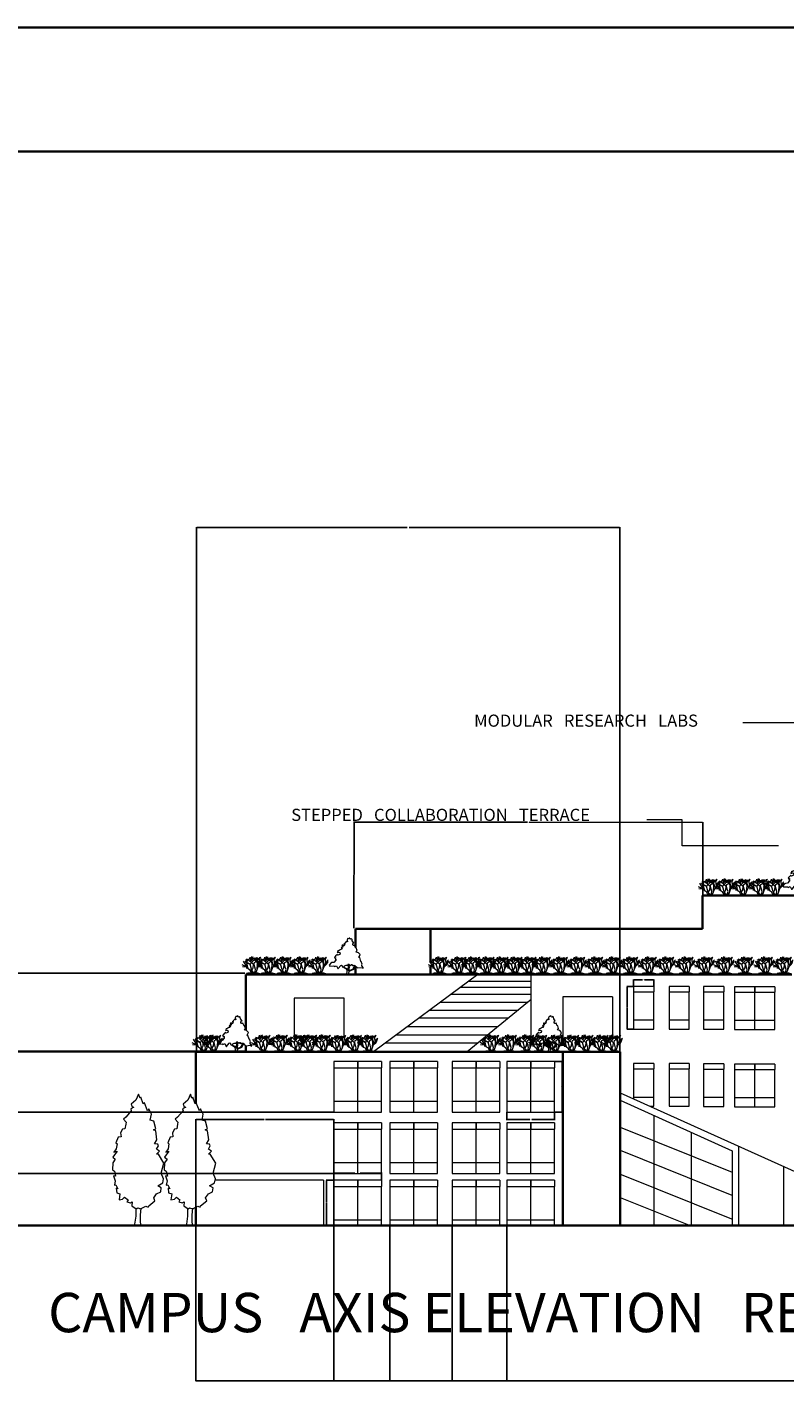
# Model space of a CAD drawing. Units: inches. Extents: x -934 to 898, y -1502 to 444.
# Tile 7 of 10: x -511 to -117, y -270 to 444. Entities that reach past the tile are written whole.
import ezdxf

# ---------------------------------------------------------------- set-up
doc = ezdxf.new("R2010")
doc.units = ezdxf.units.IN
doc.header["$MEASUREMENT"] = 0
for name, color, linetype, lineweight in [('A-ANNO-DIMS', 2, 'Continuous', 18), ('A-ANNO-TEXT', 7, 'Continuous', 18), ('A-ANNO-TITL', 7, 'Continuous', 30), ('A-ANNO-TTLB', 7, 'Continuous', 35), ('A-ELEV', 7, 'Continuous', 35), ('A-FLOR-STRS', 7, 'Continuous', 18), ('A-GLAZ', 4, 'Continuous', 13), ('L-GRND', 7, 'Continuous', 35), ('L-PLNT-TREE', 3, 'Continuous', 13)]:
    doc.layers.add(name, color=color, linetype=linetype, lineweight=lineweight)
doc.styles.get("Standard").update_dxf_attribs({"font": 'arial.ttf'})
doc.dimstyles.get("Standard").update_dxf_attribs({"dimtxt": 0.18, "dimasz": 0.18, "dimexe": 0.18, "dimexo": 0.0625, "dimgap": 0.09, "dimtad": 0, "dimtih": 1, "dimtoh": 1, "dimdec": 4, "dimzin": 0, "dimdsep": 46, "dimtxsty": 'Standard', "dimcen": 0.09, "dimadec": 0, "dimazin": 0, "dimtfac": 1, "dimtdec": 4, "dimtofl": 0, "dimtmove": 0, "dimatfit": 3, "dimfxl": 1, "dimtolj": 1, "dimtzin": 0, "dimarcsym": 0})

# ---------------------------------------------------------------- blocks, each defined once
blk = doc.blocks.new('*U2')
for points in [[(22.0124, 137.721), (18.5475, 141.5624), (15.5282, 138.2446), (13.8028, 139.3505), (13.3714, 142.1153), (11.2148, 143.2214), (8.1954, 140.4564), (4.7447, 141.0094), (2.1567, 136.0326), (2.1567, 131.6088), (5.6074, 129.9499), (3.0193, 128.2909), (0.4313, 130.5029), (-6.9015, 123.3141), (-6.9015, 121.6552), (-9.9208, 119.9963), (-9.0581, 118.3373), (-6.9015, 115.0195), (-10.7835, 112.2546), (-14.6656, 115.0195), (-16.8222, 114.4665), (-17.6849, 112.2546), (-14.6656, 111.7016), (-14.2342, 107.2778), (-17.6065, 107.8307), (-21.5669, 103.9599), (-17.2536, 103.4069), (-18.9789, 97.8771), (-22.8609, 97.3241), (-27.1743, 94.5593), (-32.3504, 91.7944), (-32.7817, 94.0063), (-36.6638, 85.7116), (-29.7624, 87.3705), (-25.449, 84.6056), (-26.743, 77.9699), (-34.507, 75.205), (-37.9578, 77.4169), (-39.2518, 74.099), (-42.2711, 73.5461), (-44.8592, 70.2282), (-47.8786, 66.3574), (-43.9965, 63.0395), (-41.4085, 64.6985), (-44.3346, 59.8898), (-42.2089, 60.1377), (-42.5159, 55.7849), (-49.6039, 46.4502), (-58.2307, 45.8972), (-62.1127, 43.6853), (-68.5828, 36.4966), (-65.9947, 32.0727), (-50.0352, 32.6257), (-47.0159, 30.4138), (-39.6831, 33.7317), (-34.507, 22.6721), (-32.3504, 22.6721), (-22.4296, 34.8376), (-19.4102, 36.4966), (-17.2536, 33.7317), (-17.2536, 29.8608), (-13.8028, 28.7549), (-9.0581, 28.7549), (-7.3328, 32.6257), (-1.7254, 35.3906), (3.8821, 35.9436), (6.4701, 38.1555), (6.9014, 38.7085), (8.1954, 41.4734), (9.9208, 40.3674), (11.2148, 35.9436), (14.2341, 37.6025), (15.0968, 36.4966), (15.9595, 33.7317), (18.9789, 38.7085), (21.9982, 38.7085), (23.2922, 36.4966), (21.9982, 34.2847), (25.4489, 35.3906), (26.743, 33.7317), (29.7623, 35.9436), (32.7817, 34.8376), (38.8204, 28.7549), (41.4084, 27.6489), (43.5651, 25.437), (61.6813, 27.0959), (65.132, 23.7781), (67.7201, 24.884), (60.8186, 33.7317), (60.3873, 37.0495), (62.544, 40.3674), (58.662, 50.874), (56.5053, 50.874), (52.1919, 66.3574), (47.8785, 66.9103), (50.4665, 69.1222), (53.9172, 77.9699), (47.0158, 85.1586), (38.3891, 87.9235), (42.2711, 94.0063)], [(42.2711, 94.0063), (38.8204, 104.5129), (36.6637, 104.5129), (32.3503, 113.9135), (29.7623, 113.3605), (26.743, 113.3605), (24.5862, 117.7844), (25.8802, 123.8671), (29.331, 123.8671), (22.8609, 131.6088), (21.9982, 137.6916)], [(-12.9401, 28.7549), (-2.588, 22.1191), (0.8626, 17.6953), (1.7253, 11.6125), (0, 0)], [(-9.9208, 28.2019), (0, 23.2251), (3.4507, 19.9072), (4.7447, 15.4834), (8.6267, 27.0959), (6.4701, 37.6025)], [(34.5071, 33.1787), (27.1743, 18.2483), (9.0581, 10.5066), (7.7641, 3.8708), (8.1954, 0)], [(8.1954, 40.3674), (11.2148, 27.6489), (8.1954, 13.8245), (24.5862, 19.9072), (32.7817, 34.2847)]]:
    blk.add_lwpolyline(points)
blk = doc.blocks.new('*U5')
blk.add_lwpolyline([(-2.754, 191.699), (-6.78, 182.851), (-13.682, 176.953), (-11.956, 173.266), (-9.656, 172.529), (-14.257, 170.317), (-13.682, 167.368), (-21.733, 157.783), (-25.184, 154.834), (-21.158, 150.41), (-21.733, 147.461), (-22.884, 140.825), (-26.334, 140.087), (-29.21, 134.926), (-28.635, 129.028), (-32.661, 128.291), (-36.111, 120.18), (-34.386, 118.706), (-35.536, 111.333), (-38.987, 106.171), (-34.386, 107.646), (-40.712, 98.798), (-37.261, 95.849), (-40.712, 90.688), (-41.287, 80.366), (-38.412, 78.154), (-36.686, 70.781), (-39.562, 71.518), (-37.261, 64.145), (-38.412, 57.509), (-36.111, 58.247), (-33.236, 52.348), (-35.536, 53.086), (-34.961, 46.45), (-30.36, 44.975), (-31.51, 36.128), (-26.334, 36.865), (-23.459, 39.814), (-18.283, 36.128), (-20.008, 33.178), (-14.832, 31.704), (-11.956, 33.178), (-12.531, 27.28), (-6.205, 22.856), (-3.905, 24.331), (0.121, 22.856), (8.173, 26.543), (11.624, 25.068), (12.199, 27.28), (21.4, 34.653), (19.675, 39.077), (23.701, 44.975), (30.027, 47.924), (30.602, 53.823), (25.426, 56.772), (32.903, 61.196), (34.053, 67.094), (30.602, 75.205), (34.628, 89.951), (26.576, 103.222), (23.701, 103.222), (28.302, 107.646), (23.701, 110.595), (26.576, 115.756), (25.426, 117.968), (20.825, 118.706), (24.276, 124.604), (22.551, 137.876), (19.1, 139.35), (22.551, 140.825), (19.675, 151.884), (14.499, 153.359), (16.224, 162.207), (12.199, 170.317), (10.473, 167.368), (5.872, 179.165), (4.147, 177.69), (0.696, 187.275), (-0.454, 185.8)], close=True)
for points in [[(-6.813, 23.669), (-6.813, 11.669), (-8.627, 0)], [(0.387, 23.669), (-0.576, 13.271), (-0.576, 3.686), (0, 0)]]:
    blk.add_lwpolyline(points)
blk = doc.blocks.new('*U6')
for p, q in [((-426.72, 414.528), (-475.488, 475.488)), ((-377.952, 463.296), (-451.104, 487.68)), ((-426.72, 414.528), (-390.144, 499.872)), ((-377.952, 463.296), (-329.184, 524.256)), ((-316.7634, 502.285), (-327.6092, 559.9176)), ((-296.5958, 484.4034), (-316.7634, 502.285)), ((-286.512, 498.3226), (-307.4416, 538.0736)), ((-305.8922, 396.9512), (-302.7934, 478.4344)), ((-302.7934, 478.4344), (-270.256, 518.1854)), ((-290.3982, 464.5406), (-265.6078, 577.8246)), ((-268.7066, 458.5716), (-250.0884, 500.3038)), ((-207.264, 451.104), (-268.224, 548.64)), ((-240.792, 502.285), (-228.3968, 573.8368)), ((-182.88, 499.872), (-219.456, 512.064)), ((-207.264, 451.104), (-134.112, 487.68)), ((-182.88, 499.872), (-158.496, 536.448)), ((-121.92, 414.528), (-182.88, 499.872)), ((-129.1844, 450.6214), (-140.0302, 542.036)), ((-134.112, 487.68), (-97.536, 548.64)), ((-73.152, 329.184), (-109.728, 499.872)), ((-97.536, 426.72), (-24.384, 524.256)), ((-85.7758, 472.4908), (-73.3552, 548.005)), ((-70.2564, 426.7708), (-85.7758, 472.4908)), ((-73.152, 402.336), (-60.96, 512.064)), ((-12.9032, 555.9552), (-2.0574, 522.1732)), ((-5.1562, 486.3846), (2.5908, 542.036)), ((8.7884, 335.3562), (-5.1562, 486.3846)), ((-3.6068, 492.3536), (14.986, 518.1854)), ((-0.508, 508.254), (22.7584, 536.067)), ((1.0414, 526.1356), (35.1536, 559.9176)), ((2.5908, 542.036), (21.209, 555.9552)), ((-451.104, 219.456), (-601.0402, 303.8094)), ((-451.104, 219.456), (-587.4512, 234.2388)), ((-463.296, 280.416), (-552.577, 423.037)), ((-463.296, 280.416), (-512.064, 292.608)), ((-329.184, 316.992), (-499.872, 414.528)), ((-353.568, 316.992), (-487.68, 377.952)), ((-402.336, 207.264), (-463.296, 280.416)), ((-414.528, 182.88), (-463.296, 182.88)), ((-426.72, 316.992), (-451.104, 329.184)), ((-377.952, 146.304), (-451.104, 219.456)), ((-402.336, 12.192), (-451.104, 0)), ((-426.72, 316.992), (-426.72, 414.528)), ((-402.336, 207.264), (-426.72, 316.992)), ((-377.952, 146.304), (-402.336, 207.264)), ((-341.376, 12.192), (-402.336, 12.192)), ((-207.264, 304.8), (-377.952, 463.296)), ((-329.184, 121.92), (-377.952, 146.304)), ((-329.184, 316.992), (-353.568, 316.992)), ((-243.84, 24.384), (-341.376, 12.192)), ((-338.455, 424.7896), (-290.3982, 464.5406)), ((-329.184, 316.992), (-207.264, 451.104)), ((-268.224, 109.728), (-329.184, 316.992)), ((-292.608, 60.96), (-329.184, 121.92)), ((-243.84, 24.384), (-329.184, 0)), ((-304.3428, 426.7708), (-268.7066, 458.5716)), ((-219.456, 24.384), (-292.608, 60.96)), ((-268.224, 109.728), (-219.456, 195.072)), ((-219.456, 48.768), (-268.224, 109.728)), ((-243.84, 24.384), (-195.072, 24.384)), ((-219.456, 195.072), (-207.264, 304.8)), ((-219.456, 24.384), (-109.728, 73.152)), ((-219.456, 24.384), (-158.496, 73.152)), ((-219.456, 24.384), (-219.456, 48.768)), ((-219.456, 24.384), (-73.152, 24.384)), ((-195.072, 316.992), (-182.88, 377.952)), ((-170.688, 219.456), (-195.072, 316.992)), ((-195.072, 24.384), (-158.496, 12.192)), ((-182.88, 377.952), (-97.536, 426.72)), ((-146.304, 134.112), (-170.688, 219.456)), ((-158.496, 73.152), (-146.304, 134.112)), ((-158.496, 12.192), (-85.344, 0)), ((-85.7758, 389.001), (-129.1844, 452.6026)), ((-109.728, 73.152), (-48.768, 243.84)), ((-85.344, 134.112), (-73.152, 329.184)), ((-24.384, 268.224), (-73.152, 402.336)), ((-73.152, 24.384), (0, 0)), ((-48.768, 243.84), (24.384, 304.8)), ((-12.192, 274.32), (8.7884, 335.3562)), ((8.7884, 335.3562), (33.6042, 412.8516)), ((24.384, 304.8), (36.576, 390.144)), ((24.384, 304.8), (73.152, 377.952)), ((33.6042, 412.8516), (92.5068, 464.5406)), ((36.576, 390.144), (73.152, 438.912)), ((48.768, 341.376), (60.96, 390.144)), ((60.96, 390.144), (85.344, 414.528))]:
    blk.add_line(p, q)
blk = doc.blocks.new('WIN-TWIN-WIDE')
for p, q in [((12.45, 26.32), (0, 26.32)), ((0, 26.32), (0, 23.06)), ((0, 23.06), (0, 5.73)), ((0, 23.06), (12.45, 23.06)), ((24.78, 26.32), (12.34, 26.32)), ((12.34, 26.32), (12.34, 23.06)), ((12.34, 23.06), (12.34, 5.73)), ((12.34, 23.06), (24.78, 23.06)), ((12.45, 26.32), (12.45, 23.06)), ((12.45, 5.73), (12.45, 23.06)), ((24.78, 26.32), (24.78, 23.06)), ((24.78, 5.73), (24.78, 23.06)), ((0, 5.73), (12.45, 5.73)), ((0, 5.73), (0, 0)), ((0, 0), (12.45, 0)), ((12.34, 5.73), (24.78, 5.73)), ((12.34, 5.73), (12.34, 0)), ((12.34, 0), (24.78, 0)), ((12.45, 0), (12.45, 5.73)), ((24.78, 0), (24.78, 5.73))]:
    blk.add_line(p, q)
blk = doc.blocks.new('WIN-TWIN-NARROW')
for p, q in [((10.5, 22.21), (0, 22.21)), ((0, 22.21), (0, 19.45)), ((20.91, 22.21), (10.41, 22.21)), ((10.41, 22.21), (10.41, 19.45)), ((10.5, 22.21), (10.5, 19.45)), ((20.91, 22.21), (20.91, 19.45)), ((0, 19.45), (0, 4.84)), ((0, 19.45), (10.5, 19.45)), ((10.41, 19.45), (10.41, 4.84)), ((10.41, 19.45), (20.91, 19.45)), ((10.5, 4.84), (10.5, 19.45)), ((20.91, 4.84), (20.91, 19.45)), ((0, 4.84), (10.5, 4.84)), ((0, 4.84), (0, 0)), ((0, 0), (10.5, 0)), ((10.41, 4.84), (20.91, 4.84)), ((10.41, 4.84), (10.41, 0)), ((10.41, 0), (20.91, 0)), ((10.5, 0), (10.5, 4.84)), ((20.91, 0), (20.91, 4.84))]:
    blk.add_line(p, q)
blk = doc.blocks.new('WIN-TWIN-AT-GRADE')
for p, q in [((12.45, 23.64), (0, 23.64)), ((0, 23.64), (0, 20.37)), ((24.78, 23.64), (12.34, 23.64)), ((12.34, 23.64), (12.34, 20.37)), ((12.45, 23.64), (12.45, 20.37)), ((24.78, 23.64), (24.78, 20.37)), ((0, 20.37), (0, 3.04)), ((0, 20.37), (12.45, 20.37)), ((12.34, 20.37), (12.34, 3.04)), ((12.34, 20.37), (24.78, 20.37)), ((12.45, 3.04), (12.45, 20.37)), ((24.78, 3.04), (24.78, 20.37)), ((0, 3.04), (12.45, 3.04)), ((0, 3.04), (0, 0)), ((12.34, 3.04), (24.78, 3.04)), ((12.34, 3.04), (12.34, 0)), ((12.45, 0), (12.45, 3.04)), ((24.78, 0), (24.78, 3.04))]:
    blk.add_line(p, q)
blk = doc.blocks.new('WIN-SINGLE-NARROW')
for p, q in [((10.5, 22.21), (0, 22.21)), ((0, 22.21), (0, 19.45)), ((10.5, 22.21), (10.5, 19.45)), ((0, 19.45), (0, 4.84)), ((0, 19.45), (10.5, 19.45)), ((10.5, 4.84), (10.5, 19.45)), ((0, 4.84), (10.5, 4.84)), ((0, 4.84), (0, 0)), ((0, 0), (10.5, 0)), ((10.5, 0), (10.5, 4.84))]:
    blk.add_line(p, q)
blk = doc.blocks.new('*D31')
at = {"layer": 'A-ANNO-DIMS', "color": 0, "lineweight": -2, "transparency": 16777216}
for p, q in [((-236.7, -93.3), (-232.64, -93.3)), ((-232.82, -93.48), (-232.82, -106.28)), ((-232.82, -119.44), (-232.82, -106.64)), ((-236.7, -119.62), (-232.64, -119.62))]:
    blk.add_line(p, q, dxfattribs=at)
at = {"layer": 'A-ANNO-DIMS', "color": 0, "transparency": 16777216}
for points in [[(-232.85, -93.48), (-232.79, -93.48), (-232.82, -93.3)], [(-232.85, -119.44), (-232.79, -119.44), (-232.82, -119.62)]]:
    blk.add_solid(points, dxfattribs=at)
at = {"layer": 'Defpoints', "color": 0, "transparency": 16777216}
for p in [(-236.77, -93.3), (-232.82, -93.3), (-236.77, -119.62)]:
    blk.add_point(p, dxfattribs=at)
at = {"layer": 'A-ANNO-DIMS', "color": 0, "transparency": 16777216, "insert": (-232.82, -106.46), "char_height": 0.18, "attachment_point": 5}
blk.add_mtext('\\A1;TWIN 26 TYP.', dxfattribs=at)
blk = doc.blocks.new('*D32')
at = {"layer": 'A-ANNO-DIMS', "color": 0, "lineweight": -2, "transparency": 16777216}
for p, q in [((-261.55, -119.69), (-261.55, -123.75)), ((-236.77, -119.69), (-236.77, -123.75)), ((-261.37, -123.57), (-249.69, -123.57)), ((-236.95, -123.57), (-248.63, -123.57))]:
    blk.add_line(p, q, dxfattribs=at)
at = {"layer": 'A-ANNO-DIMS', "color": 0, "transparency": 16777216}
for points in [[(-261.37, -123.54), (-261.37, -123.6), (-261.55, -123.57)], [(-236.95, -123.54), (-236.95, -123.6), (-236.77, -123.57)]]:
    blk.add_solid(points, dxfattribs=at)
at = {"layer": 'Defpoints', "color": 0, "transparency": 16777216}
for p in [(-261.55, -119.62), (-236.77, -119.62), (-236.77, -123.57)]:
    blk.add_point(p, dxfattribs=at)
at = {"layer": 'A-ANNO-DIMS', "color": 0, "transparency": 16777216, "insert": (-249.16, -123.57), "char_height": 0.18, "attachment_point": 5}
blk.add_mtext('\\A1;25 TYP.', dxfattribs=at)
blk = doc.blocks.new('*D33')
at = {"layer": 'A-ANNO-DIMS', "color": 0, "lineweight": -2, "transparency": 16777216}
for p, q in [((-351.59, -154.98), (-351.59, -151.14)), ((-351.41, -151.32), (-340.56, -151.32)), ((-326.98, -151.32), (-337.83, -151.32)), ((-326.8, -154.98), (-326.8, -151.14))]:
    blk.add_line(p, q, dxfattribs=at)
at = {"layer": 'A-ANNO-DIMS', "color": 0, "transparency": 16777216}
for points in [[(-351.41, -151.29), (-351.41, -151.35), (-351.59, -151.32)], [(-326.98, -151.29), (-326.98, -151.35), (-326.8, -151.32)]]:
    blk.add_solid(points, dxfattribs=at)
at = {"layer": 'Defpoints', "color": 0, "transparency": 16777216}
for p in [(-351.59, -155.04), (-326.8, -151.32), (-326.8, -155.04)]:
    blk.add_point(p, dxfattribs=at)
at = {"layer": 'A-ANNO-DIMS', "color": 0, "transparency": 16777216, "insert": (-339.19, -151.32), "char_height": 0.18, "attachment_point": 5}
blk.add_mtext('\\A1;GRADE TWIN 25 TYP.', dxfattribs=at)
blk = doc.blocks.new('*D34')
at = {"layer": 'A-ANNO-DIMS', "color": 0, "lineweight": -2, "transparency": 16777216}
for p, q in [((-351.65, -155.04), (-355.48, -155.04)), ((-355.3, -155.22), (-355.3, -166.68)), ((-355.3, -178.5), (-355.3, -167.04)), ((-351.65, -178.68), (-355.48, -178.68))]:
    blk.add_line(p, q, dxfattribs=at)
at = {"layer": 'A-ANNO-DIMS', "color": 0, "transparency": 16777216}
for points in [[(-355.33, -155.22), (-355.27, -155.22), (-355.3, -155.04)], [(-355.33, -178.5), (-355.27, -178.5), (-355.3, -178.68)]]:
    blk.add_solid(points, dxfattribs=at)
at = {"layer": 'Defpoints', "color": 0, "transparency": 16777216}
for p in [(-355.3, -155.04), (-351.59, -155.04), (-351.59, -178.68)]:
    blk.add_point(p, dxfattribs=at)
at = {"layer": 'A-ANNO-DIMS', "color": 0, "transparency": 16777216, "insert": (-355.3, -166.86), "char_height": 0.18, "attachment_point": 5}
blk.add_mtext('\\A1;24 TYP.', dxfattribs=at)
blk = doc.blocks.new('*D37')
at = {"layer": 'A-ANNO-DIMS', "color": 0, "lineweight": -2, "transparency": 16777216}
for p, q in [((-195.8, -54.27), (-199.25, -54.27)), ((-199.07, -54.45), (-199.07, -65.19)), ((-199.07, -76.29), (-199.07, -65.55)), ((-195.8, -76.47), (-199.25, -76.47))]:
    blk.add_line(p, q, dxfattribs=at)
at = {"layer": 'A-ANNO-DIMS', "color": 0, "transparency": 16777216}
for points in [[(-199.1, -54.45), (-199.04, -54.45), (-199.07, -54.27)], [(-199.1, -76.29), (-199.04, -76.29), (-199.07, -76.47)]]:
    blk.add_solid(points, dxfattribs=at)
at = {"layer": 'Defpoints', "color": 0, "transparency": 16777216}
for p in [(-199.07, -54.27), (-195.74, -54.27), (-195.74, -76.47)]:
    blk.add_point(p, dxfattribs=at)
at = {"layer": 'A-ANNO-DIMS', "color": 0, "transparency": 16777216, "insert": (-199.07, -65.37), "char_height": 0.18, "attachment_point": 5}
blk.add_mtext('\\A1;SINGLE 22 TYP.', dxfattribs=at)
blk = doc.blocks.new('*D38')
at = {"layer": 'A-ANNO-DIMS', "color": 0, "lineweight": -2, "transparency": 16777216}
for p, q in [((-195.74, -54.2), (-195.74, -50.75)), ((-195.56, -50.93), (-191.01, -50.93)), ((-185.42, -50.93), (-189.97, -50.93)), ((-185.24, -54.2), (-185.24, -50.75))]:
    blk.add_line(p, q, dxfattribs=at)
at = {"layer": 'A-ANNO-DIMS', "color": 0, "transparency": 16777216}
for points in [[(-195.56, -50.9), (-195.56, -50.96), (-195.74, -50.93)], [(-185.42, -50.9), (-185.42, -50.96), (-185.24, -50.93)]]:
    blk.add_solid(points, dxfattribs=at)
at = {"layer": 'Defpoints', "color": 0, "transparency": 16777216}
for p in [(-195.74, -54.27), (-185.24, -50.93), (-185.24, -54.27)]:
    blk.add_point(p, dxfattribs=at)
at = {"layer": 'A-ANNO-DIMS', "color": 0, "transparency": 16777216, "insert": (-190.49, -50.93), "char_height": 0.18, "attachment_point": 5}
blk.add_mtext('\\A1;11 TYP.', dxfattribs=at)
blk = doc.blocks.new('*D79')
at = {"layer": 'A-ANNO-DIMS', "color": 0, "lineweight": -2, "transparency": 16777216}
for p, q in [((278.23, -122.09), (278.23, -259.51)), ((-423.28, -178.74), (-423.28, -259.51)), ((-423.1, -259.33), (-72.92, -259.33)), ((278.05, -259.33), (-72.13, -259.33))]:
    blk.add_line(p, q, dxfattribs=at)
at = {"layer": 'A-ANNO-DIMS', "color": 0, "transparency": 16777216}
for points in [[(-423.1, -259.3), (-423.1, -259.36), (-423.28, -259.33)], [(278.05, -259.3), (278.05, -259.36), (278.23, -259.33)]]:
    blk.add_solid(points, dxfattribs=at)
at = {"layer": 'Defpoints', "color": 0, "transparency": 16777216}
for p in [(278.23, -122.02), (-423.28, -178.68), (278.23, -259.33)]:
    blk.add_point(p, dxfattribs=at)
at = {"layer": 'A-ANNO-DIMS', "color": 0, "transparency": 16777216, "insert": (-72.53, -259.33), "char_height": 0.18, "attachment_point": 5}
blk.add_mtext('\\A1;701.5', dxfattribs=at)
blk = doc.blocks.new('*D81')
at = {"layer": 'A-ANNO-DIMS', "color": 0, "lineweight": -2, "transparency": 16777216}
for p, q in [((-422.93, -88.17), (-422.93, 184.53)), ((-422.75, 184.35), (-313.38, 184.35)), ((-203.07, 184.35), (-312.45, 184.35)), ((-202.89, -88.16), (-202.89, 184.53))]:
    blk.add_line(p, q, dxfattribs=at)
at = {"layer": 'A-ANNO-DIMS', "color": 0, "transparency": 16777216}
for points in [[(-422.75, 184.38), (-422.75, 184.32), (-422.93, 184.35)], [(-203.07, 184.38), (-203.07, 184.32), (-202.89, 184.35)]]:
    blk.add_solid(points, dxfattribs=at)
at = {"layer": 'Defpoints', "color": 0, "transparency": 16777216}
for p in [(-202.89, 184.35), (-422.93, -88.23), (-202.89, -88.23)]:
    blk.add_point(p, dxfattribs=at)
at = {"layer": 'A-ANNO-DIMS', "color": 0, "transparency": 16777216, "insert": (-312.91, 184.35), "char_height": 0.18, "attachment_point": 5}
blk.add_mtext('\\A1;220.04', dxfattribs=at)
blk = doc.blocks.new('*D84')
at = {"layer": 'A-ANNO-DIMS', "color": 0, "lineweight": -2, "transparency": 16777216}
for p, q in [((-423, -88.23), (-628.55, -88.23)), ((-628.37, -88.41), (-628.37, -133.27)), ((-628.37, -178.5), (-628.37, -133.64)), ((-423.34, -178.68), (-628.55, -178.68))]:
    blk.add_line(p, q, dxfattribs=at)
at = {"layer": 'A-ANNO-DIMS', "color": 0, "transparency": 16777216}
for points in [[(-628.4, -88.41), (-628.34, -88.41), (-628.37, -88.23)], [(-628.4, -178.5), (-628.34, -178.5), (-628.37, -178.68)]]:
    blk.add_solid(points, dxfattribs=at)
at = {"layer": 'Defpoints', "color": 0, "transparency": 16777216}
for p in [(-628.37, -88.23), (-422.93, -88.23), (-423.28, -178.68)]:
    blk.add_point(p, dxfattribs=at)
at = {"layer": 'A-ANNO-DIMS', "color": 0, "transparency": 16777216, "insert": (-628.37, -133.45), "char_height": 0.18, "attachment_point": 5}
blk.add_mtext('\\A1;90.45', dxfattribs=at)
blk = doc.blocks.new('*D85')
at = {"layer": 'A-ANNO-DIMS', "color": 0, "lineweight": -2, "transparency": 16777216}
for p, q in [((-397.86, -47.36), (-628.55, -47.36)), ((-628.37, -47.54), (-628.37, -67.5)), ((-628.37, -87.82), (-628.37, -67.86)), ((-397.99, -88), (-628.55, -88))]:
    blk.add_line(p, q, dxfattribs=at)
at = {"layer": 'A-ANNO-DIMS', "color": 0, "transparency": 16777216}
for points in [[(-628.4, -47.54), (-628.34, -47.54), (-628.37, -47.36)], [(-628.4, -87.82), (-628.34, -87.82), (-628.37, -88)]]:
    blk.add_solid(points, dxfattribs=at)
at = {"layer": 'Defpoints', "color": 0, "transparency": 16777216}
for p in [(-628.37, -47.36), (-397.8, -47.36), (-397.93, -88)]:
    blk.add_point(p, dxfattribs=at)
at = {"layer": 'A-ANNO-DIMS', "color": 0, "transparency": 16777216, "insert": (-628.37, -67.68), "char_height": 0.18, "attachment_point": 5}
blk.add_mtext('\\A1;40.63', dxfattribs=at)
blk = doc.blocks.new('*D88')
at = {"layer": 'A-ANNO-DIMS', "color": 0, "lineweight": -2, "transparency": 16777216}
for p, q in [((-341.11, -23.96), (-341.02, 31.41)), ((-340.84, 31.23), (-250.81, 31.09)), ((-159.87, 30.95), (-249.9, 31.09)), ((-159.77, -24.24), (-159.69, 31.13))]:
    blk.add_line(p, q, dxfattribs=at)
at = {"layer": 'A-ANNO-DIMS', "color": 0, "transparency": 16777216}
for points in [[(-340.84, 31.26), (-340.84, 31.2), (-341.02, 31.23)], [(-159.87, 30.98), (-159.87, 30.92), (-159.69, 30.95)]]:
    blk.add_solid(points, dxfattribs=at)
at = {"layer": 'Defpoints', "color": 0, "transparency": 16777216}
for p in [(-159.69, 30.95), (-341.11, -24.02), (-159.77, -24.3)]:
    blk.add_point(p, dxfattribs=at)
at = {"layer": 'A-ANNO-DIMS', "color": 0, "transparency": 16777216, "insert": (-250.36, 31.09), "char_height": 0.18, "attachment_point": 5}
blk.add_mtext('\\A1;181.34', dxfattribs=at)
blk = doc.blocks.new('*D91')
at = {"layer": 'A-ANNO-DIMS', "color": 0, "lineweight": -2, "transparency": 16777216}
for p, q in [((-423.28, -178.62), (-423.28, -123.25)), ((-423.1, -123.43), (-387.76, -123.43)), ((-351.77, -123.43), (-387.11, -123.43)), ((-351.59, -178.62), (-351.59, -123.25))]:
    blk.add_line(p, q, dxfattribs=at)
at = {"layer": 'A-ANNO-DIMS', "color": 0, "transparency": 16777216}
for points in [[(-423.1, -123.4), (-423.1, -123.46), (-423.28, -123.43)], [(-351.77, -123.4), (-351.77, -123.46), (-351.59, -123.43)]]:
    blk.add_solid(points, dxfattribs=at)
at = {"layer": 'Defpoints', "color": 0, "transparency": 16777216}
for p in [(-351.59, -123.43), (-423.28, -178.68), (-351.59, -178.68)]:
    blk.add_point(p, dxfattribs=at)
at = {"layer": 'A-ANNO-DIMS', "color": 0, "transparency": 16777216, "insert": (-387.43, -123.43), "char_height": 0.18, "attachment_point": 5}
blk.add_mtext('\\A1;71.7', dxfattribs=at)
blk = doc.blocks.new('*D92')
at = {"layer": 'A-ANNO-DIMS', "color": 0, "lineweight": -2, "transparency": 16777216}
for p, q in [((-351.59, -178.74), (-351.59, -259.51)), ((-322.47, -178.74), (-322.47, -259.51)), ((-351.41, -259.33), (-337.49, -259.33)), ((-322.65, -259.33), (-336.56, -259.33))]:
    blk.add_line(p, q, dxfattribs=at)
at = {"layer": 'A-ANNO-DIMS', "color": 0, "transparency": 16777216}
for points in [[(-351.41, -259.3), (-351.41, -259.36), (-351.59, -259.33)], [(-322.65, -259.3), (-322.65, -259.36), (-322.47, -259.33)]]:
    blk.add_solid(points, dxfattribs=at)
at = {"layer": 'Defpoints', "color": 0, "transparency": 16777216}
for p in [(-351.59, -178.68), (-322.47, -178.68), (-322.47, -259.33)]:
    blk.add_point(p, dxfattribs=at)
at = {"layer": 'A-ANNO-DIMS', "color": 0, "transparency": 16777216, "insert": (-337.03, -259.33), "char_height": 0.18, "attachment_point": 5}
blk.add_mtext('\\A1;29.113', dxfattribs=at)
blk = doc.blocks.new('*D93')
at = {"layer": 'A-ANNO-DIMS', "color": 0, "lineweight": -2, "transparency": 16777216}
for p, q in [((-322.47, -178.74), (-322.47, -259.51)), ((-289.97, -178.74), (-289.97, -259.51)), ((-322.29, -259.33), (-306.68, -259.33)), ((-290.15, -259.33), (-305.76, -259.33))]:
    blk.add_line(p, q, dxfattribs=at)
at = {"layer": 'A-ANNO-DIMS', "color": 0, "transparency": 16777216}
for points in [[(-322.29, -259.3), (-322.29, -259.36), (-322.47, -259.33)], [(-290.15, -259.3), (-290.15, -259.36), (-289.97, -259.33)]]:
    blk.add_solid(points, dxfattribs=at)
at = {"layer": 'Defpoints', "color": 0, "transparency": 16777216}
for p in [(-322.47, -178.68), (-289.97, -178.68), (-289.97, -259.33)]:
    blk.add_point(p, dxfattribs=at)
at = {"layer": 'A-ANNO-DIMS', "color": 0, "transparency": 16777216, "insert": (-306.22, -259.33), "char_height": 0.18, "attachment_point": 5}
blk.add_mtext('\\A1;32.505', dxfattribs=at)
blk = doc.blocks.new('*D94')
at = {"layer": 'A-ANNO-DIMS', "color": 0, "lineweight": -2, "transparency": 16777216}
for p, q in [((-289.97, -178.74), (-289.97, -259.51)), ((-261.55, -178.74), (-261.55, -259.51)), ((-289.79, -259.33), (-276.23, -259.33)), ((-261.73, -259.33), (-275.29, -259.33))]:
    blk.add_line(p, q, dxfattribs=at)
at = {"layer": 'A-ANNO-DIMS', "color": 0, "transparency": 16777216}
for points in [[(-289.79, -259.3), (-289.79, -259.36), (-289.97, -259.33)], [(-261.73, -259.3), (-261.73, -259.36), (-261.55, -259.33)]]:
    blk.add_solid(points, dxfattribs=at)
at = {"layer": 'Defpoints', "color": 0, "transparency": 16777216}
for p in [(-289.97, -178.68), (-261.55, -178.68), (-261.55, -259.33)]:
    blk.add_point(p, dxfattribs=at)
at = {"layer": 'A-ANNO-DIMS', "color": 0, "transparency": 16777216, "insert": (-275.76, -259.33), "char_height": 0.18, "attachment_point": 5}
blk.add_mtext('\\A1;28.415', dxfattribs=at)
blk = doc.blocks.new('*D95')
at = {"layer": 'A-ANNO-DIMS', "color": 0, "lineweight": -2, "transparency": 16777216}
for p, q in [((-351.65, -151.52), (-628.55, -151.52)), ((-628.37, -151.7), (-628.37, -164.92)), ((-628.37, -178.5), (-628.37, -165.28)), ((-351.65, -178.68), (-628.55, -178.68))]:
    blk.add_line(p, q, dxfattribs=at)
at = {"layer": 'A-ANNO-DIMS', "color": 0, "transparency": 16777216}
for points in [[(-628.4, -151.7), (-628.34, -151.7), (-628.37, -151.52)], [(-628.4, -178.5), (-628.34, -178.5), (-628.37, -178.68)]]:
    blk.add_solid(points, dxfattribs=at)
at = {"layer": 'Defpoints', "color": 0, "transparency": 16777216}
for p in [(-628.37, -151.52), (-351.59, -151.52), (-351.59, -178.68)]:
    blk.add_point(p, dxfattribs=at)
at = {"layer": 'A-ANNO-DIMS', "color": 0, "transparency": 16777216, "insert": (-628.37, -165.1), "char_height": 0.18, "attachment_point": 5}
blk.add_mtext('\\A1;27.16', dxfattribs=at)
blk = doc.blocks.new('*D96')
at = {"layer": 'A-ANNO-DIMS', "color": 0, "lineweight": -2, "transparency": 16777216}
for p, q in [((-351.65, -119.62), (-628.55, -119.62)), ((-628.37, -119.8), (-628.37, -135.39)), ((-628.37, -151.34), (-628.37, -135.75)), ((-351.65, -151.52), (-628.55, -151.52))]:
    blk.add_line(p, q, dxfattribs=at)
at = {"layer": 'A-ANNO-DIMS', "color": 0, "transparency": 16777216}
for points in [[(-628.4, -119.8), (-628.34, -119.8), (-628.37, -119.62)], [(-628.4, -151.34), (-628.34, -151.34), (-628.37, -151.52)]]:
    blk.add_solid(points, dxfattribs=at)
at = {"layer": 'Defpoints', "color": 0, "transparency": 16777216}
for p in [(-628.37, -119.62), (-351.59, -119.62), (-351.59, -151.52)]:
    blk.add_point(p, dxfattribs=at)
at = {"layer": 'A-ANNO-DIMS', "color": 0, "transparency": 16777216, "insert": (-628.37, -135.57), "char_height": 0.18, "attachment_point": 5}
blk.add_mtext('\\A1;31.89', dxfattribs=at)

msp = doc.modelspace()

# ---------------------------------------------------------------- linework, layer by layer
at = {"layer": 'A-ANNO-TEXT'}
for p, q in [((-104.1148, 82.8773), (-138.836, 82.8773)), ((-170.3558, 32.3925), (-188.8841, 32.3925)), ((-170.3558, 18.9224), (-170.3558, 32.3925)), ((-120.416, 18.9224), (-170.3558, 18.9224))]:
    msp.add_line(p, q, dxfattribs=at)
at = {"layer": 'A-ANNO-TTLB'}
for points in [[(-933.5092, 444.4646), (897.7239, 444.4646), (897.7239, -1501.5858), (-933.5092, -1501.5858)], [(-892.081, 380.0228), (832.9871, 380.0228), (832.9871, -1448.0237), (-892.081, -1448.0237)]]:
    msp.add_lwpolyline(points, close=True, dxfattribs=at)
at = {"layer": 'A-ELEV'}
for p, q in [((-159.7746, -7.0768), (-159.7746, -24.3023)), ((20.5463, -7.0768), (-159.7746, -7.0768)), ((-340.3117, -24.3023), (-340.3117, -33.8561)), ((-301.278, -24.3023), (-340.3117, -24.3023)), ((-159.7746, -24.3023), (-302.7187, -24.3023)), ((-301.278, -24.3023), (-301.278, -41.7664)), ((-301.278, -41.7664), (-301.278, -24.3023)), ((-113.3269, -47.999), (-397.2277, -47.999)), ((-397.2277, -47.999), (-397.2277, -77.1423)), ((-340.3117, -43.7182), (-340.3117, -47.999)), ((-340.3117, -45.1475), (-340.3117, -47.0067)), ((-301.278, -47.999), (-301.278, -44.1299)), ((-301.278, -44.1299), (-301.278, -47.999)), ((-397.2277, -85.1028), (-397.2277, -88.3005)), ((-423.2792, -88.3005), (-203.1303, -88.3005)), ((-423.2792, -114.9148), (-423.2792, -88.3005)), ((-346.2559, -88.3005), (-346.2559, -88.2047)), ((-232.4714, -88.3005), (-232.4714, -178.6804)), ((-202.6582, -88.3005), (-211.4299, -88.3005)), ((-202.6582, -88.3005), (-203.1303, -88.3005)), ((-202.6582, -88.3005), (-202.6582, -178.6804)), ((-423.2792, -178.6804), (-423.2792, -169.0547))]:
    msp.add_line(p, q, dxfattribs=at)
at = {"layer": 'A-FLOR-STRS'}
for p, q in [((-276.6245, -47.999), (-330.9093, -88.3005)), ((-248.919, -82.8992), (-248.919, -47.999)), ((-285.6829, -54.724), (-248.919, -54.724)), ((-281.3842, -51.5327), (-248.919, -51.5327)), ((-296.0314, -62.4068), (-250.5022, -62.4068)), ((-290.6183, -58.3881), (-248.919, -58.3881)), ((-248.919, -61.1146), (-282.227, -88.3005)), ((-307.0205, -70.5653), (-260.4979, -70.5653)), ((-301.6468, -66.5757), (-255.6099, -66.5757)), ((-313.1061, -75.0833), (-266.0334, -75.0833)), ((-324.5802, -83.6017), (-276.4701, -83.6017)), ((-319.077, -79.5161), (-271.4644, -79.5161)), ((-248.919, -88.3005), (-248.919, -87.8829)), ((-202.6582, -109.6295), (-49.5955, -178.6804)), ((-202.6582, -113.4293), (-144.5024, -139.7546)), ((-185.2363, -121.3156), (-185.2363, -178.6804)), ((-202.6582, -127.455), (-144.5024, -150.827)), ((-165.7493, -130.1368), (-165.7493, -178.6804)), ((-202.693, -139.4704), (-144.5373, -162.8423)), ((-144.5024, -135.7193), (-144.5024, -135.8652)), ((-144.5024, -139.7546), (-144.5024, -178.6804)), ((-141.1983, -137.3558), (-141.1983, -178.6804)), ((-117.73, -147.943), (-117.73, -178.6804)), ((-203.0191, -151.7032), (-144.8634, -175.0751)), ((-202.6582, -164.0718), (-166.3081, -178.6804))]:
    msp.add_line(p, q, dxfattribs=at)
at = {"layer": 'A-GLAZ'}
for p, q in [((-346.2559, -60.3894), (-372.1394, -60.3894)), ((-372.1394, -60.3894), (-372.1394, -79.87)), ((-346.2559, -80.4454), (-346.2559, -60.3894)), ((-206.5879, -59.7434), (-232.4714, -59.7434)), ((-232.4714, -59.7434), (-232.4714, -81.759)), ((-206.5879, -59.7434), (-206.5879, -81.955)), ((-372.1394, -81.4917), (-372.1394, -81.839)), ((-372.1394, -83.2295), (-372.1394, -83.5562)), ((-346.2559, -84.6701), (-346.2559, -83.8696)), ((-206.5879, -87.6789), (-206.5879, -87.8562)), ((-185.2363, -94.4294), (-195.7388, -94.4294)), ((-195.7388, -94.4294), (-195.7388, -97.1843)), ((-195.7388, -97.1843), (-195.7388, -111.8026)), ((-195.7388, -97.1843), (-185.2363, -97.1843)), ((-185.2363, -94.4294), (-185.2363, -97.1843)), ((-185.2363, -111.8026), (-185.2363, -97.1843)), ((-195.7388, -111.8026), (-185.2363, -111.8026)), ((-195.7388, -111.8026), (-195.7388, -112.7511)), ((-185.2363, -116.638), (-185.2363, -111.8026)), ((-187.1228, -116.638), (-185.2363, -116.638)), ((-356.9247, -151.5178), (-414.3018, -151.5178)), ((-356.9247, -155.0427), (-413.2757, -155.0427)), ((-356.9247, -151.5178), (-351.5859, -151.5178)), ((-356.9247, -155.0427), (-356.9247, -178.6804))]:
    msp.add_line(p, q, dxfattribs=at)
at = {"layer": 'L-GRND'}
msp.add_line((284.8904, -178.6804), (-573.1189, -178.6804), dxfattribs=at)

# ---------------------------------------------------------------- block references
at = {"layer": 'A-GLAZ'}
for name, p in [('WIN-SINGLE-NARROW', (-195.7388, -76.4745)), ('WIN-SINGLE-NARROW', (-177.2524, -76.4745)), ('WIN-SINGLE-NARROW', (-159.2942, -76.4745)), ('WIN-TWIN-NARROW', (-143.2139, -76.7521)), ('WIN-TWIN-WIDE', (-351.5859, -119.6248)), ('WIN-TWIN-WIDE', (-322.4726, -119.6248)), ('WIN-TWIN-WIDE', (-289.9675, -119.6248)), ('WIN-TWIN-WIDE', (-261.552, -119.6248)), ('WIN-SINGLE-NARROW', (-177.2524, -116.638)), ('WIN-SINGLE-NARROW', (-159.2942, -116.6847)), ('WIN-TWIN-NARROW', (-143.2139, -116.9623)), ('WIN-TWIN-WIDE', (-351.5859, -151.5178)), ('WIN-TWIN-WIDE', (-322.4726, -151.5178)), ('WIN-TWIN-WIDE', (-289.9675, -151.5178)), ('WIN-TWIN-WIDE', (-261.552, -151.5178)), ('WIN-TWIN-AT-GRADE', (-351.5859, -178.6804)), ('WIN-TWIN-AT-GRADE', (-322.4726, -178.6804)), ('WIN-TWIN-AT-GRADE', (-289.9675, -178.6804)), ('WIN-TWIN-AT-GRADE', (-261.552, -178.6804))]:
    msp.add_blockref(name, p, dxfattribs=at)
at = {"layer": 'L-PLNT-TREE'}
for name, p, xscale, yscale, zscale in [('*U2', (-109.0605, -6.747), 0.1315554675521508, 0.1315554675521508, 0.1315554675521508), ('*U6', (-152.7689, -7.0221), 0.0152219259934872, 0.0152219259934872, 0.0152219259934872), ('*U6', (-144.3676, -7.0221), 0.0152219259934872, 0.0152219259934872, 0.0152219259934872), ('*U6', (-135.5978, -7.0221), 0.0152219259934872, 0.0152219259934872, 0.0152219259934872), ('*U6', (-126.6629, -7.0221), 0.0152219259934872, 0.0152219259934872, 0.0152219259934872), ('*U6', (-118.9248, -7.0221), 0.0152219259934872, 0.0152219259934872, 0.0152219259934872), ('*U2', (-344.9801, -47.9429), 0.1315554675521508, 0.1315554675521508, 0.1315554675521508), ('*U6', (-390.0805, -47.5966), 0.0152219259934872, 0.0152219259934872, 0.0152219259934872), ('*U6', (-382.4315, -47.5966), 0.0152219259934872, 0.0152219259934872, 0.0152219259934872), ('*U6', (-374.185, -47.5966), 0.0152219259934872, 0.0152219259934872, 0.0152219259934872), ('*U6', (-365.3409, -47.5966), 0.0152219259934872, 0.0152219259934872, 0.0152219259934872), ('*U6', (-355.862, -47.5966), 0.0152219259934872, 0.0152219259934872, 0.0152219259934872), ('*U6', (-293.2481, -47.5966), 0.0152219259934872, 0.0152219259934872, 0.0152219259934872), ('*U6', (-283.3262, -47.5966), 0.0152219259934872, 0.0152219259934872, 0.0152219259934872), ('*U6', (-276.2167, -47.5966), 0.0152219259934872, 0.0152219259934872, 0.0152219259934872), ('*U6', (-268.6778, -47.5966), 0.0152219259934872, 0.0152219259934872, 0.0152219259934872), ('*U6', (-261.4113, -47.5966), 0.0152219259934872, 0.0152219259934872, 0.0152219259934872), ('*U6', (-254.1587, -47.5966), 0.0152219259934872, 0.0152219259934872, 0.0152219259934872), ('*U6', (-246.9061, -47.5966), 0.0152219259934872, 0.0152219259934872, 0.0152219259934872), ('*U6', (-239.3912, -47.5966), 0.0152219259934872, 0.0152219259934872, 0.0152219259934872), ('*U6', (-230.5163, -47.5966), 0.0152219259934872, 0.0152219259934872, 0.0152219259934872), ('*U6', (-221.4982, -47.5966), 0.0152219259934872, 0.0152219259934872, 0.0152219259934872), ('*U6', (-212.1819, -47.5966), 0.0152219259934872, 0.0152219259934872, 0.0152219259934872), ('*U6', (-203.0684, -47.5966), 0.0152219259934872, 0.0152219259934872, 0.0152219259934872), ('*U6', (-193.9893, -47.5966), 0.0152219259934872, 0.0152219259934872, 0.0152219259934872), ('*U6', (-184.351, -47.5966), 0.0152219259934872, 0.0152219259934872, 0.0152219259934872), ('*U6', (-175.2684, -47.5966), 0.0152219259934872, 0.0152219259934872, 0.0152219259934872), ('*U6', (-165.1904, -47.5966), 0.0152219259934872, 0.0152219259934872, 0.0152219259934872), ('*U6', (-154.9795, -47.5966), 0.0152219259934872, 0.0152219259934872, 0.0152219259934872), ('*U6', (-144.7569, -47.5966), 0.0152219259934872, 0.0152219259934872, 0.0152219259934872), ('*U6', (-134.4028, -47.5966), 0.0152219259934872, 0.0152219259934872, 0.0152219259934872), ('*U6', (-123.9399, -47.5966), 0.0152219259934872, 0.0152219259934872, 0.0152219259934872), ('*U6', (-114.1107, -47.5966), 0.0152219259934872, 0.0152219259934872, 0.0152219259934872), ('*U2', (-403.0601, -88.4584), 0.1315554675521508, 0.1315554675521508, 0.1315554675521508), ('*U2', (-240.2422, -88.4584), 0.1315554675521508, 0.1315554675521508, 0.1315554675521508), ('*U6', (-416.0677, -88.2276), 0.0152219259934872, 0.0152219259934872, 0.0152219259934872), ('*U6', (-410.8287, -88.2276), 0.0152219259934872, 0.0152219259934872, 0.0152219259934872), ('*U6', (-385.1809, -88.2276), 0.0152219259934872, 0.0152219259934872, 0.0152219259934872), ('*U6', (-376.1884, -88.1346), 0.0152219259934872, 0.0152219259934872, 0.0152219259934872), ('*U6', (-367.2012, -88.1346), 0.0152219259934872, 0.0152219259934872, 0.0152219259934872), ('*U6', (-360.9141, -88.1346), 0.0152219259934872, 0.0152219259934872, 0.0152219259934872), ('*U6', (-353.8411, -88.1346), 0.0152219259934872, 0.0152219259934872, 0.0152219259934872), ('*U6', (-345.8265, -88.3479), 0.0152219259934872, 0.0152219259934872, 0.0152219259934872), ('*U6', (-337.6267, -88.2017), 0.0152219259934872, 0.0152219259934872, 0.0152219259934872), ('*U6', (-330.1209, -88.2017), 0.0152219259934872, 0.0152219259934872, 0.0152219259934872), ('*U6', (-266.3486, -88.1522), 0.0152219259934872, 0.0152219259934872, 0.0152219259934872), ('*U6', (-257.0437, -88.1522), 0.0152219259934872, 0.0152219259934872, 0.0152219259934872), ('*U6', (-248.1111, -88.1522), 0.0152219259934872, 0.0152219259934872, 0.0152219259934872), ('*U6', (-241.2504, -88.1522), 0.0152219259934872, 0.0152219259934872, 0.0152219259934872), ('*U6', (-233.1926, -88.2274), 0.0152219259934872, 0.0152219259934872, 0.0152219259934872), ('*U6', (-224.682, -88.2274), 0.0152219259934872, 0.0152219259934872, 0.0152219259934872), ('*U6', (-217.2564, -88.2274), 0.0152219259934872, 0.0152219259934872, 0.0152219259934872), ('*U6', (-209.3814, -88.2274), 0.0152219259934872, 0.0152219259934872, 0.0152219259934872), ('*U6', (-202.8927, -88.2274), 0.0152219259934872, 0.0152219259934872, 0.0152219259934872), ('*U5', (-452.1002, -177.9527), 0.3528399638811642, 0.3528399638811642, 0.3528399638811642), ('*U5', (-425.1421, -177.9527), 0.3528399638811642, 0.3528399638811642, 0.3528399638811642)]:
    msp.add_blockref(name, p, dxfattribs=dict(at, xscale=xscale, yscale=yscale, zscale=zscale))

# ---------------------------------------------------------------- texts
at = {"layer": 'A-ANNO-TEXT'}
for s, p in [('MODULAR   RESEARCH   LABS ', (-278.598, 80.7933)), ('STEPPED   COLLABORATION   TERRACE', (-373.7034, 31.7977))]:
    msp.add_text(s, height=6.31231, dxfattribs=at).set_placement(p)
at = {"layer": 'A-ANNO-TITL'}
msp.add_text('LINEAR   CAMPUS   AXIS ELEVATION   RESEARCH   AND   INNOVATION   SPINE ', height=20.457511, dxfattribs=at).set_placement((-613.4854, -234.1138))

# ---------------------------------------------------------------- dimensions: what is measured, and where the dimension line sits
at = {"layer": 'A-ANNO-DIMS'}
for base, p1, p2, override, picture, middle in [((-202.8927, 184.3524), (-422.9344, -88.2276), (-202.8927, -88.2274), {"dimdec": 2, "dimlfac": 1, "dimrnd": 0, "dimzin": 0, "dimdsep": 46, "dimlunit": 2}, '*D81', (-312.9135, 184.3524)), ((278.229, -259.3312), (-423.2792, -178.6804), (278.229, -122.024), {"dimdec": 1, "dimlfac": 1, "dimrnd": 0, "dimzin": 0, "dimdsep": 46, "dimlunit": 2}, '*D79', (-72.5251, -259.3312)), ((-322.4726, -259.3312), (-351.5859, -178.6804), (-322.4726, -178.6804), {"dimdec": 3, "dimlfac": 1, "dimrnd": 0, "dimzin": 0, "dimdsep": 46, "dimlunit": 2}, '*D92', (-337.0292, -259.3312)), ((-289.9675, -259.3312), (-322.4726, -178.6804), (-289.9675, -178.6804), {"dimdec": 3, "dimlfac": 1, "dimrnd": 0, "dimzin": 0, "dimdsep": 46, "dimlunit": 2}, '*D93', (-306.22, -259.3312)), ((-261.55202, -259.33121), (-289.96747, -178.68037), (-261.55202, -178.68037), {"dimdec": 3, "dimlfac": 1, "dimrnd": 0, "dimzin": 0, "dimdsep": 46, "dimlunit": 2}, '*D94', (-275.75975, -259.33121))]:
    dim = msp.add_linear_dim(base=base, p1=p1, p2=p2, dimstyle='Standard', override=override, dxfattribs=at)
    dim.commit()
    dim.dimension.update_dxf_attribs({"geometry": picture, "text_midpoint": middle})
for base, p1, p2, angle, override, picture, middle in [((-159.6889, 30.9477), (-341.1099, -24.0211), (-159.7746, -24.3023), 359.9111626, {"dimdec": 2, "dimlfac": 1, "dimrnd": 0, "dimzin": 0, "dimdsep": 46, "dimlunit": 2}, '*D88', (-250.3565, 31.0883)), ((-628.3689, -47.3642), (-397.9256, -87.9953), (-397.7996, -47.3642), 90, {"dimdec": 2, "dimlfac": 1, "dimrnd": 0, "dimzin": 0, "dimdsep": 46, "dimlunit": 2}, '*D85', (-628.3689, -67.6798)), ((-628.3689, -88.2276), (-423.2792, -178.6804), (-422.9344, -88.2276), 90, {"dimdec": 2, "dimlfac": 1, "dimrnd": 0, "dimzin": 0, "dimdsep": 46, "dimlunit": 2}, '*D84', (-628.3689, -133.454)), ((-628.3689, -119.6248), (-351.5859, -151.5178), (-351.5859, -119.6248), 90, {"dimdec": 2, "dimlfac": 1, "dimrnd": 0, "dimzin": 0, "dimdsep": 46, "dimlunit": 2}, '*D96', (-628.3689, -135.5713)), ((-351.5859, -123.4304), (-423.2792, -178.6804), (-351.5859, -178.6804), 0, {"dimdec": 1, "dimlfac": 1, "dimrnd": 0, "dimzin": 0, "dimdsep": 46, "dimlunit": 2}, '*D91', (-387.4325, -123.4304)), ((-628.3689, -151.5178), (-351.5859, -178.6804), (-351.5859, -151.5178), 90, {"dimdec": 2, "dimlfac": 1, "dimrnd": 0, "dimzin": 0, "dimdsep": 46, "dimlunit": 2}, '*D95', (-628.3689, -165.0991))]:
    dim = msp.add_linear_dim(base=base, p1=p1, p2=p2, angle=angle, dimstyle='Standard', override=override, dxfattribs=at)
    dim.commit()
    dim.dimension.update_dxf_attribs({"geometry": picture, "text_midpoint": middle})
for base, p1, p2, text, picture, middle in [((-199.0701, -54.2659), (-195.7388, -76.4745), (-195.7388, -54.2659), 'SINGLE <> TYP.', '*D37', (-199.0701, -65.3702)), ((-232.8186, -93.3007), (-236.7672, -119.6248), (-236.7672, -93.3007), 'TWIN <> TYP.', '*D31', (-232.8186, -106.4628)), ((-355.3036, -155.0427), (-351.5859, -178.6804), (-351.5859, -155.0427), '<> TYP.', '*D34', (-355.3036, -166.8615))]:
    dim = msp.add_linear_dim(base=base, p1=p1, p2=p2, angle=90, text=text, dimstyle='Standard', override={"dimdec": 0, "dimlfac": 1, "dimrnd": 0, "dimzin": 0, "dimdsep": 46, "dimlunit": 2}, dxfattribs=at)
    dim.commit()
    dim.dimension.update_dxf_attribs({"geometry": picture, "text_midpoint": middle})
for base, p1, p2, text, picture, middle in [((-185.2363, -50.9346), (-195.7388, -54.2659), (-185.2363, -54.2659), '<> TYP.', '*D38', (-190.4875, -50.9346)), ((-236.7672, -123.5735), (-261.552, -119.6248), (-236.7672, -119.6248), '<> TYP.', '*D32', (-249.1596, -123.5735)), ((-326.801, -151.325), (-351.5859, -155.0427), (-326.801, -155.0427), 'GRADE TWIN <> TYP.', '*D33', (-339.1934, -151.325))]:
    dim = msp.add_linear_dim(base=base, p1=p1, p2=p2, text=text, dimstyle='Standard', override={"dimdec": 0, "dimlfac": 1, "dimrnd": 0, "dimzin": 0, "dimdsep": 46, "dimlunit": 2}, dxfattribs=at)
    dim.commit()
    dim.dimension.update_dxf_attribs({"geometry": picture, "text_midpoint": middle})

doc.saveas('drawing.dxf')
